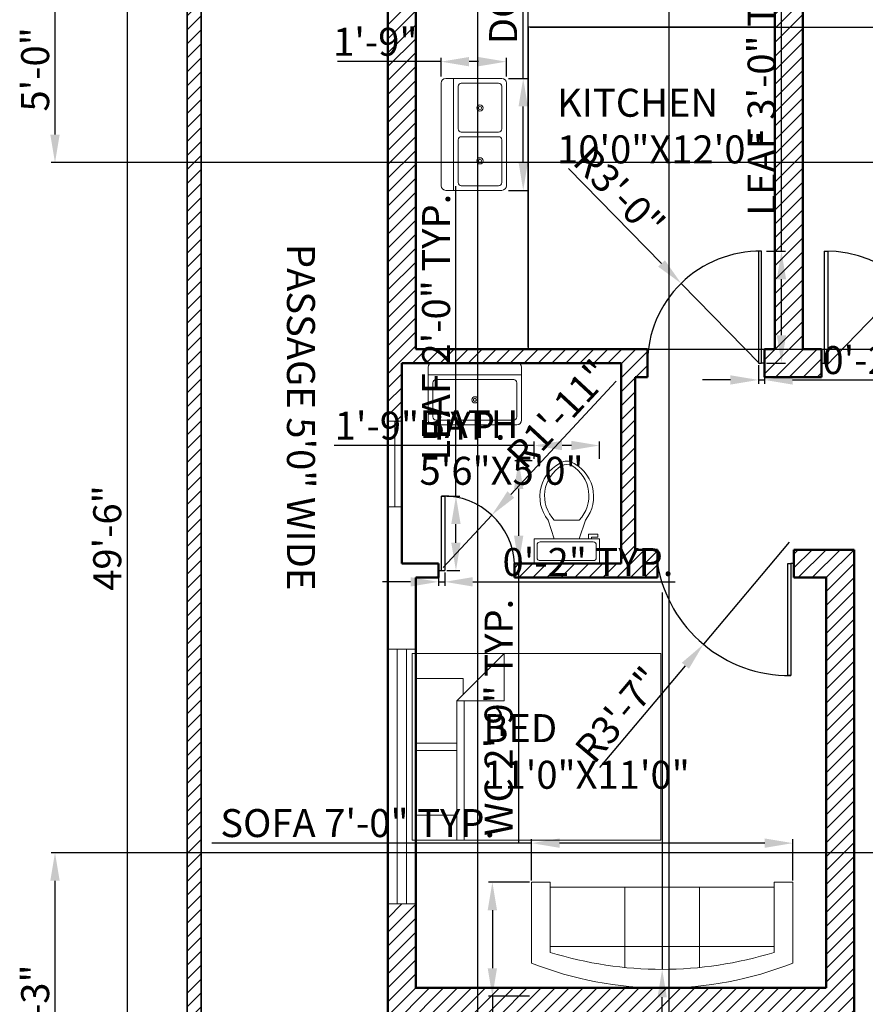
# Model space of a CAD drawing. Units: inches. Extents: x 36184 to 36805, y 18177 to 19069.
# Tile 3 of 5: x 36191 to 36463, y 18560 to 18876. Entities that reach past the tile are written whole.
import ezdxf

# ---------------------------------------------------------------- set-up
doc = ezdxf.new("R2010")
doc.units = ezdxf.units.IN
for name, color, linetype, lineweight in [('A-ANNO-DIMS', 2, 'Continuous', 18), ('A-AREA-IDEN', 7, 'Continuous', 25), ('A-DOOR', 4, 'Continuous', 25), ('A-FLOR-CASE', 9, 'Continuous', 25), ('A-FLOR-FIXT', 9, 'Continuous', 18), ('A-FURN', 8, 'Continuous', 18), ('A-GLAZ', 4, 'Continuous', 18), ('A-WALL', 7, 'Continuous', 50), ('C-PROP', 7, 'Continuous', 35), ('L-SITE-WALL', 7, 'Continuous', 35)]:
    doc.layers.add(name, color=color, linetype=linetype, lineweight=lineweight)
doc.layers.add('A-WALL-PATT', color=244, linetype='Continuous', lineweight=13, true_color=0x991b1e)
doc.styles.get("Standard").update_dxf_attribs({"font": 'arial.ttf'})
doc.dimstyles.new('ISO-25', dxfattribs={"dimtxt": 9, "dimasz": 9, "dimexe": 1.25, "dimexo": 0.625, "dimtad": 1, "dimdec": 1, "dimrnd": 9, "dimlunit": 3, "dimtxsty": 'Standard', "dimcen": 2.5, "dimadec": 0, "dimazin": 0, "dimtfac": 1, "dimtdec": 1, "dimtmove": 0, "dimatfit": 3, "dimfxl": 1, "dimarcsym": 0})

# ---------------------------------------------------------------- blocks, each defined once
blk = doc.blocks.new('Sink-double - 36 in top')
for p, q in [((-18, -4), (18, -4)), ((-0.75, -18.5), (-0.75, -6.5)), ((0.75, -6.5), (0.75, -18.5))]:
    blk.add_line(p, q)
for points in [[(-16.5, 0), (16.5, 0)], [(-18, -19.5), (-18, -1.5)], [(18, -1.5), (18, -19.5)], [(-15.5, -5.5), (-1.75, -5.5)], [(1.75, -5.5), (15.5, -5.5)], [(-16.5, -18.5), (-16.5, -6.5)], [(16.5, -6.5), (16.5, -18.5)], [(16.5, -21), (-16.5, -21)], [(-1.75, -19.5), (-15.5, -19.5)], [(15.5, -19.5), (1.75, -19.5)]]:
    blk.add_lwpolyline(points)
for centre, radius in [((-8.5, -12.5), 1), ((-8.5, -12.5), 0.5), ((8.5, -12.5), 1), ((8.5, -12.5), 0.5)]:
    blk.add_circle(centre, radius)
for centre, radius, start, end in [((-16.5, -1.5), 1.5, 90, 180), ((16.5, -1.5), 1.5, 0, 90), ((-15.5, -6.5), 1, 90, 180), ((-1.75, -6.5), 1, 0, 90), ((1.75, -6.5), 1, 90, 180), ((15.5, -6.5), 1, 0, 90), ((-15.5, -18.5), 1, 180, 270), ((-1.75, -18.5), 1, 270, 0), ((1.75, -18.5), 1, 180, 270), ((15.5, -18.5), 1, 270, 0), ((-16.5, -19.5), 1.5, 180, 270), ((16.5, -19.5), 1.5, 270, 0)]:
    blk.add_arc(centre, radius, start, end)
blk = doc.blocks.new('Sofa - Roundback 7 ft.')
for p, q in [((-12.00002, -32.4421), (-12.00003, -6.5971)), ((11.99997, -32.4421), (11.99998, -6.5971)), ((-36.000027, -34), (-36.000027, -11.4696)), ((35.99998, -34), (35.99998, -11.4696)), ((-35.999844, -13.3819), (35.9998, -13.3819)), ((-36.000027, -32.4421), (35.99998, -32.4421))]:
    blk.add_line(p, q)
for points in [[(-36.000027, -34), (-42.000027, -34), (-42.000027, -8)], [(41.99998, -8), (41.99998, -34), (35.99998, -34)]]:
    blk.add_lwpolyline(points)
for centre, radius, start, end in [((0, -114.25), 114.25, 68.43141, 111.5686), ((-0.00001, -127.1968), 121.1968, 72.72033, 107.2797)]:
    blk.add_arc(centre, radius, start, end)
blk = doc.blocks.new('Bed - Queen')
for p, q in [((0, -80.00003), (0, 0)), ((0, 0), (59.99999, 0)), ((59.99999, 0), (59.99999, -80.00003)), ((7.99999, -1.2), (28.79998, -1.2)), ((7.99999, -14.4), (7.99999, -1.2)), ((28.79998, -1.2), (28.79998, -14.4)), ((31.19999, -1.2), (51.99999, -1.2)), ((31.19999, -14.4), (31.19999, -1.2)), ((51.99999, -1.2), (51.99999, -16.4)), ((0, -14.4), (44.8, -14.4)), ((59.99999, -29.6), (44.8, -14.4)), ((44.8, -14.4), (44.8, -29.6)), ((44.8, -16.8), (0, -16.8)), ((51.99999, -16.4), (46.79936, -16.4)), ((44.8, -29.6), (59.99999, -29.6)), ((59.99999, -80.00003), (0, -80.00003))]:
    blk.add_line(p, q)
blk = doc.blocks.new('Toilet - top')
for p, q in [((9.5, -6), (9.5, -2)), ((-10, -8.5), (-8, -8.5)), ((-10, -9.5), (-10, -8.5)), ((-7, -9.5), (-10, -9.5)), ((-8, -8.5), (-8, -8)), ((-7, -8), (-7, -9.5)), ((-4, -8), (-6, -14)), ((4, -8), (6, -14)), ((4, -14), (-4, -14))]:
    blk.add_line(p, q)
blk.add_lwpolyline([(10.5, -8), (10.5, 0), (-10.5, 0), (-10.5, -8)], close=True)
for points in [[(-9.5, -2), (-9.5, -6)], [(8.5, -1), (-8.5, -1)], [(-8.5, -7), (8.5, -7)]]:
    blk.add_lwpolyline(points)
for centre, radius, start, end in [((-8.62, -1.88), 0.884, 81.8699, 188.1301), ((8.62, -1.88), 0.884, 351.8699, 98.1301), ((-8.62, -6.12), 0.884, 171.8699, 278.1301), ((8.62, -6.12), 0.884, 261.8699, 8.1301), ((3.52, -21.58), 12.17, 141.4691, 247.9714), ((4.2, -21.82), 11.33, 136.3677, 238.9468), ((-3.52, -21.58), 12.17, 292.0284, 38.5307), ((-4.2, -21.82), 11.33, 301.053, 43.6321), ((0, -27.88), 4, 245.7318, 294.2682), ((0, -29), 4, 254.8605, 285.1395)]:
    blk.add_arc(centre, radius, start, end)
blk = doc.blocks.new('Sink-single - 30 in top')
blk.add_line((-15, -3.999996), (15, -3.999996))
for points in [[(-13.5, 0), (13.5, 0)], [(-15, -18.499996), (-15, -1.5)], [(15, -1.5), (15, -18.499996)], [(-12.5, -5.499996), (12.5, -5.499996)], [(-13.5, -17.499996), (-13.5, -6.499996)], [(13.5, -6.499996), (13.5, -17.499996)], [(12.5, -18.499996), (-12.5, -18.499996)], [(13.5, -19.999996), (-13.5, -19.999996)]]:
    blk.add_lwpolyline(points)
for radius in [1, 0.5]:
    blk.add_circle((0, -11.999996), radius)
for centre, radius, start, end in [((-13.5, -1.5), 1.5, 90, 180), ((13.5, -1.5), 1.5, 0, 90), ((-12.5, -6.499996), 1, 90, 180), ((12.5, -6.499996), 1, 0, 90), ((-13.5, -18.499996), 1.5, 180, 270), ((-12.5, -17.499996), 1, 180, 270), ((12.5, -17.499996), 1, 270, 0), ((13.5, -18.499996), 1.5, 270, 0)]:
    blk.add_arc(centre, radius, start, end)
blk = doc.blocks.new('*D14')
at = {"layer": 'A-ANNO-DIMS', "color": 0, "lineweight": -2, "transparency": 16777216}
for p, q in [((36244.69, 19007.3), (36224.73, 19007.3)), ((36225.98, 18998.3), (36225.98, 18420.79)), ((36244.69, 18411.79), (36224.73, 18411.79))]:
    blk.add_line(p, q, dxfattribs=at)
at = {"layer": 'A-ANNO-DIMS', "color": 0, "transparency": 16777216}
for points in [[(36224.48, 18998.3), (36227.48, 18998.3), (36225.98, 19007.3)], [(36224.48, 18420.79), (36227.48, 18420.79), (36225.98, 18411.79)]]:
    blk.add_solid(points, dxfattribs=at)
at = {"layer": 'Defpoints', "color": 0, "transparency": 16777216}
for p in [(36245.31, 19007.3), (36225.98, 18411.79), (36245.31, 18411.79)]:
    blk.add_point(p, dxfattribs=at)
at = {"layer": 'A-ANNO-DIMS', "color": 0, "transparency": 16777216, "insert": (36220.76, 18709.54), "char_height": 9, "attachment_point": 5, "rotation": 90}
blk.add_mtext('49\'-6"', dxfattribs=at)
blk = doc.blocks.new('DOOR-LEAF-24IN')
for p, q in [((1, 0), (1, 24)), ((1, 24), (2, 24)), ((2, 24), (2, 0)), ((0, 0), (1, 0)), ((1, 0), (2, 0))]:
    blk.add_line(p, q)
blk = doc.blocks.new('DOOR-LEAF-36IN')
for p, q in [((1, 36), (0, 36)), ((0, 36), (0, 0)), ((1, 0), (1, 36)), ((0, 0), (1, 0)), ((2, 0), (1, 0))]:
    blk.add_line(p, q)
blk = doc.blocks.new('*D22')
at = {"layer": 'A-ANNO-DIMS', "color": 0, "lineweight": -2, "transparency": 16777216}
for p, q in [((36356.04, 18611.4), (36253.25, 18611.4)), ((36356.04, 18599.43), (36356.04, 18612.65)), ((36431.04, 18611.4), (36365.04, 18611.4)), ((36440.04, 18599.43), (36440.04, 18612.65))]:
    blk.add_line(p, q, dxfattribs=at)
at = {"layer": 'A-ANNO-DIMS', "color": 0, "transparency": 16777216}
for points in [[(36365.04, 18612.9), (36365.04, 18609.9), (36356.04, 18611.4)], [(36431.04, 18612.9), (36431.04, 18609.9), (36440.04, 18611.4)]]:
    blk.add_solid(points, dxfattribs=at)
at = {"layer": 'Defpoints', "color": 0, "transparency": 16777216}
for p in [(36356.04, 18611.4), (36356.04, 18598.8), (36440.04, 18598.8)]:
    blk.add_point(p, dxfattribs=at)
at = {"layer": 'A-ANNO-DIMS', "color": 0, "transparency": 16777216, "insert": (36300.14, 18616.68), "char_height": 9, "attachment_point": 5}
blk.add_mtext('SOFA 7\'-0" TYP.', dxfattribs=at)
blk = doc.blocks.new('*D23')
at = {"layer": 'A-ANNO-DIMS', "color": 0, "lineweight": -2, "transparency": 16777216}
for p, q in [((36355.41, 18598.8), (36342.19, 18598.8)), ((36343.44, 18589.8), (36343.44, 18571.14)), ((36355.41, 18562.14), (36342.19, 18562.14)), ((36343.44, 18562.14), (36343.44, 18476.06))]:
    blk.add_line(p, q, dxfattribs=at)
at = {"layer": 'A-ANNO-DIMS', "color": 0, "transparency": 16777216}
for points in [[(36341.94, 18589.8), (36344.94, 18589.8), (36343.44, 18598.8)], [(36341.94, 18571.14), (36344.94, 18571.14), (36343.44, 18562.14)]]:
    blk.add_solid(points, dxfattribs=at)
at = {"layer": 'Defpoints', "color": 0, "transparency": 16777216}
for p in [(36356.04, 18598.8), (36343.44, 18562.14), (36356.04, 18562.14)]:
    blk.add_point(p, dxfattribs=at)
at = {"layer": 'A-ANNO-DIMS', "color": 0, "transparency": 16777216, "insert": (36338.16, 18514.6), "char_height": 9, "attachment_point": 5, "rotation": 90}
blk.add_mtext('3\'-0 1/2" TYP.', dxfattribs=at)
blk = doc.blocks.new('*D26')
at = {"layer": 'A-ANNO-DIMS', "color": 0, "lineweight": -2, "transparency": 16777216}
for p, q in [((36331.73, 18723.05), (36331.73, 18822.7)), ((36328.75, 18723.05), (36332.98, 18723.05)), ((36331.73, 18708.05), (36331.73, 18714.05)), ((36328.75, 18699.05), (36332.98, 18699.05))]:
    blk.add_line(p, q, dxfattribs=at)
at = {"layer": 'A-ANNO-DIMS', "color": 0, "transparency": 16777216}
for points in [[(36330.23, 18714.05), (36333.23, 18714.05), (36331.73, 18723.05)], [(36330.23, 18708.05), (36333.23, 18708.05), (36331.73, 18699.05)]]:
    blk.add_solid(points, dxfattribs=at)
at = {"layer": 'Defpoints', "color": 0, "transparency": 16777216}
for p in [(36328.13, 18723.05), (36331.73, 18723.05), (36328.13, 18699.05)]:
    blk.add_point(p, dxfattribs=at)
at = {"layer": 'A-ANNO-DIMS', "color": 0, "transparency": 16777216, "insert": (36326.51, 18777.38), "char_height": 9, "attachment_point": 5, "rotation": 90}
blk.add_mtext('LEAF 2\'-0" TYP.', dxfattribs=at)
blk = doc.blocks.new('*D27')
at = {"layer": 'A-ANNO-DIMS', "color": 0, "lineweight": -2, "transparency": 16777216}
for p, q in [((36326.13, 18698.43), (36326.13, 18694.2)), ((36328.13, 18698.43), (36328.13, 18694.2)), ((36317.13, 18695.45), (36308.13, 18695.45)), ((36326.13, 18695.45), (36328.13, 18695.45)), ((36337.13, 18695.45), (36402.24, 18695.45))]:
    blk.add_line(p, q, dxfattribs=at)
at = {"layer": 'A-ANNO-DIMS', "color": 0, "transparency": 16777216}
for points in [[(36317.13, 18696.95), (36317.13, 18693.95), (36326.13, 18695.45)], [(36337.13, 18696.95), (36337.13, 18693.95), (36328.13, 18695.45)]]:
    blk.add_solid(points, dxfattribs=at)
at = {"layer": 'Defpoints', "color": 0, "transparency": 16777216}
for p in [(36326.13, 18699.05), (36328.13, 18699.05), (36328.13, 18695.45)]:
    blk.add_point(p, dxfattribs=at)
at = {"layer": 'A-ANNO-DIMS', "color": 0, "transparency": 16777216, "insert": (36374.18, 18700.67), "char_height": 9, "attachment_point": 5}
blk.add_mtext('0\'-2" TYP.', dxfattribs=at)
blk = doc.blocks.new('*D28')
at = {"layer": 'A-ANNO-DIMS', "color": 0, "lineweight": -2, "transparency": 16777216}
for p, q in [((36436.4, 18801.8), (36436.4, 18901.45)), ((36431.63, 18801.8), (36437.65, 18801.8)), ((36436.4, 18774.8), (36436.4, 18792.8)), ((36431.63, 18765.8), (36437.65, 18765.8))]:
    blk.add_line(p, q, dxfattribs=at)
at = {"layer": 'A-ANNO-DIMS', "color": 0, "transparency": 16777216}
for points in [[(36434.9, 18792.8), (36437.9, 18792.8), (36436.4, 18801.8)], [(36434.9, 18774.8), (36437.9, 18774.8), (36436.4, 18765.8)]]:
    blk.add_solid(points, dxfattribs=at)
at = {"layer": 'Defpoints', "color": 0, "transparency": 16777216}
for p in [(36431, 18801.8), (36436.4, 18801.8), (36431, 18765.8)]:
    blk.add_point(p, dxfattribs=at)
at = {"layer": 'A-ANNO-DIMS', "color": 0, "transparency": 16777216, "insert": (36431.18, 18856.13), "char_height": 9, "attachment_point": 5, "rotation": 90}
blk.add_mtext('LEAF 3\'-0" TYP.', dxfattribs=at)
blk = doc.blocks.new('*D29')
at = {"layer": 'A-ANNO-DIMS', "color": 0, "lineweight": -2, "transparency": 16777216}
for p, q in [((36429, 18765.18), (36429, 18759.15)), ((36431, 18765.18), (36431, 18759.15)), ((36420, 18760.4), (36411, 18760.4)), ((36429, 18760.4), (36431, 18760.4)), ((36440, 18760.4), (36505.11, 18760.4))]:
    blk.add_line(p, q, dxfattribs=at)
at = {"layer": 'A-ANNO-DIMS', "color": 0, "transparency": 16777216}
for points in [[(36420, 18761.9), (36420, 18758.9), (36429, 18760.4)], [(36440, 18761.9), (36440, 18758.9), (36431, 18760.4)]]:
    blk.add_solid(points, dxfattribs=at)
at = {"layer": 'Defpoints', "color": 0, "transparency": 16777216}
for p in [(36429, 18765.8), (36431, 18765.8), (36431, 18760.4)]:
    blk.add_point(p, dxfattribs=at)
at = {"layer": 'A-ANNO-DIMS', "color": 0, "transparency": 16777216, "insert": (36477.06, 18765.62), "char_height": 9, "attachment_point": 5}
blk.add_mtext('0\'-2" TYP.', dxfattribs=at)
blk = doc.blocks.new('*D32')
at = {"layer": 'A-ANNO-DIMS', "color": 0, "lineweight": -2, "transparency": 16777216}
for p, q in [((36356.23, 18734.35), (36350.65, 18734.35)), ((36351.9, 18725.35), (36351.9, 18710.3)), ((36356.23, 18701.3), (36350.65, 18701.3)), ((36351.9, 18701.3), (36351.9, 18611.38))]:
    blk.add_line(p, q, dxfattribs=at)
at = {"layer": 'A-ANNO-DIMS', "color": 0, "transparency": 16777216}
for points in [[(36350.4, 18725.35), (36353.4, 18725.35), (36351.9, 18734.35)], [(36350.4, 18710.3), (36353.4, 18710.3), (36351.9, 18701.3)]]:
    blk.add_solid(points, dxfattribs=at)
at = {"layer": 'Defpoints', "color": 0, "transparency": 16777216}
for p in [(36356.86, 18734.35), (36351.9, 18701.3), (36356.86, 18701.3)]:
    blk.add_point(p, dxfattribs=at)
at = {"layer": 'A-ANNO-DIMS', "color": 0, "transparency": 16777216, "insert": (36346.62, 18651.84), "char_height": 9, "attachment_point": 5, "rotation": 90}
blk.add_mtext('WC 2\'-9" TYP.', dxfattribs=at)
blk = doc.blocks.new('*D33')
at = {"layer": 'A-ANNO-DIMS', "color": 0, "lineweight": -2, "transparency": 16777216}
for p, q in [((36356.86, 18739.31), (36292.59, 18739.31)), ((36356.86, 18734.97), (36356.86, 18740.56)), ((36368.86, 18739.31), (36365.86, 18739.31)), ((36377.86, 18734.97), (36377.86, 18740.56))]:
    blk.add_line(p, q, dxfattribs=at)
at = {"layer": 'A-ANNO-DIMS', "color": 0, "transparency": 16777216}
for points in [[(36365.86, 18740.81), (36365.86, 18737.81), (36356.86, 18739.31)], [(36368.86, 18740.81), (36368.86, 18737.81), (36377.86, 18739.31)]]:
    blk.add_solid(points, dxfattribs=at)
at = {"layer": 'Defpoints', "color": 0, "transparency": 16777216}
for p in [(36356.86, 18739.31), (36356.86, 18734.35), (36377.86, 18734.35)]:
    blk.add_point(p, dxfattribs=at)
at = {"layer": 'A-ANNO-DIMS', "color": 0, "transparency": 16777216, "insert": (36320.22, 18744.53), "char_height": 9, "attachment_point": 5}
blk.add_mtext('1\'-9" TYP.', dxfattribs=at)
blk = doc.blocks.new('*D42')
at = {"layer": 'A-ANNO-DIMS', "color": 0, "lineweight": -2, "transparency": 16777216}
for p, q in [((36353.36, 18857.38), (36353.36, 18979.14)), ((36348.59, 18857.38), (36354.61, 18857.38)), ((36353.36, 18830.38), (36353.36, 18848.38)), ((36348.59, 18821.38), (36354.61, 18821.38))]:
    blk.add_line(p, q, dxfattribs=at)
at = {"layer": 'A-ANNO-DIMS', "color": 0, "transparency": 16777216}
for points in [[(36351.86, 18848.38), (36354.86, 18848.38), (36353.36, 18857.38)], [(36351.86, 18830.38), (36354.86, 18830.38), (36353.36, 18821.38)]]:
    blk.add_solid(points, dxfattribs=at)
at = {"layer": 'Defpoints', "color": 0, "transparency": 16777216}
for p in [(36347.96, 18857.38), (36353.36, 18857.38), (36347.96, 18821.38)]:
    blk.add_point(p, dxfattribs=at)
at = {"layer": 'A-ANNO-DIMS', "color": 0, "transparency": 16777216, "insert": (36348.08, 18922.76), "char_height": 9, "attachment_point": 5, "rotation": 90}
blk.add_mtext('DOUBLE SINK 3\'-0"', dxfattribs=at)
blk = doc.blocks.new('*D43')
at = {"layer": 'A-ANNO-DIMS', "color": 0, "lineweight": -2, "transparency": 16777216}
for p, q in [((36326.96, 18862.78), (36293.64, 18862.78)), ((36326.96, 18858.01), (36326.96, 18864.03)), ((36338.96, 18862.78), (36335.96, 18862.78)), ((36347.96, 18858.01), (36347.96, 18864.03))]:
    blk.add_line(p, q, dxfattribs=at)
at = {"layer": 'A-ANNO-DIMS', "color": 0, "transparency": 16777216}
for points in [[(36335.96, 18864.28), (36335.96, 18861.28), (36326.96, 18862.78)], [(36338.96, 18864.28), (36338.96, 18861.28), (36347.96, 18862.78)]]:
    blk.add_solid(points, dxfattribs=at)
at = {"layer": 'Defpoints', "color": 0, "transparency": 16777216}
for p in [(36326.96, 18862.78), (36326.96, 18857.38), (36347.96, 18857.38)]:
    blk.add_point(p, dxfattribs=at)
at = {"layer": 'A-ANNO-DIMS', "color": 0, "transparency": 16777216, "insert": (36305.8, 18868), "char_height": 9, "attachment_point": 5}
blk.add_mtext('1\'-9"', dxfattribs=at)
blk = doc.blocks.new('*D47')
at = {"layer": 'A-ANNO-DIMS', "color": 0, "lineweight": -2, "transparency": 16777216}
for p, q in [((36519.19, 18608.3), (36201.56, 18608.3)), ((36202.81, 18518.3), (36202.81, 18599.3)), ((36519.19, 18509.3), (36201.56, 18509.3))]:
    blk.add_line(p, q, dxfattribs=at)
at = {"layer": 'A-ANNO-DIMS', "color": 0, "transparency": 16777216}
for points in [[(36201.31, 18599.3), (36204.31, 18599.3), (36202.81, 18608.3)], [(36201.31, 18518.3), (36204.31, 18518.3), (36202.81, 18509.3)]]:
    blk.add_solid(points, dxfattribs=at)
at = {"layer": 'Defpoints', "color": 0, "transparency": 16777216}
for p in [(36202.81, 18608.3), (36519.81, 18608.3), (36519.81, 18509.3)]:
    blk.add_point(p, dxfattribs=at)
at = {"layer": 'A-ANNO-DIMS', "color": 0, "transparency": 16777216, "insert": (36197.59, 18558.8), "char_height": 9, "attachment_point": 5, "rotation": 90}
blk.add_mtext('8\'-3"', dxfattribs=at)
blk = doc.blocks.new('*D49')
at = {"layer": 'A-ANNO-DIMS', "color": 0, "lineweight": -2, "transparency": 16777216}
for p, q in [((36600.19, 18890.3), (36201.56, 18890.3)), ((36202.81, 18839.3), (36202.81, 18881.3)), ((36600.19, 18830.3), (36201.56, 18830.3))]:
    blk.add_line(p, q, dxfattribs=at)
at = {"layer": 'A-ANNO-DIMS', "color": 0, "transparency": 16777216}
for points in [[(36201.31, 18881.3), (36204.31, 18881.3), (36202.81, 18890.3)], [(36201.31, 18839.3), (36204.31, 18839.3), (36202.81, 18830.3)]]:
    blk.add_solid(points, dxfattribs=at)
at = {"layer": 'Defpoints', "color": 0, "transparency": 16777216}
for p in [(36202.81, 18890.3), (36600.81, 18890.3), (36600.81, 18830.3)]:
    blk.add_point(p, dxfattribs=at)
at = {"layer": 'A-ANNO-DIMS', "color": 0, "transparency": 16777216, "insert": (36197.59, 18860.3), "char_height": 9, "attachment_point": 5, "rotation": 90}
blk.add_mtext('5\'-0"', dxfattribs=at)
blk = doc.blocks.new('*D55')
at = {"layer": 'A-ANNO-DIMS', "color": 0, "lineweight": -2, "transparency": 16777216}
for p, q in [((36318.81, 18770.93), (36318.81, 19051.05)), ((36327.81, 19049.8), (36345.96, 19049.8)), ((36354.96, 18770.93), (36354.96, 19051.05))]:
    blk.add_line(p, q, dxfattribs=at)
at = {"layer": 'A-ANNO-DIMS', "color": 0, "transparency": 16777216}
for points in [[(36327.81, 19051.3), (36327.81, 19048.3), (36318.81, 19049.8)], [(36345.96, 19051.3), (36345.96, 19048.3), (36354.96, 19049.8)]]:
    blk.add_solid(points, dxfattribs=at)
at = {"layer": 'Defpoints', "color": 0, "transparency": 16777216}
for p in [(36354.96, 19049.8), (36318.81, 18770.3), (36354.96, 18770.3)]:
    blk.add_point(p, dxfattribs=at)
at = {"layer": 'A-ANNO-DIMS', "color": 0, "transparency": 16777216, "insert": (36336.89, 19055.03), "char_height": 9, "attachment_point": 5}
blk.add_mtext('3\'-0"', dxfattribs=at)
blk = doc.blocks.new('*D56')
at = {"layer": 'A-ANNO-DIMS', "color": 0, "lineweight": -2, "transparency": 16777216}
for p, q in [((36355.59, 18873.92), (36710.68, 18873.92)), ((36709.43, 18864.92), (36709.43, 18779.3)), ((36355.59, 18770.3), (36710.68, 18770.3))]:
    blk.add_line(p, q, dxfattribs=at)
at = {"layer": 'A-ANNO-DIMS', "color": 0, "transparency": 16777216}
for points in [[(36707.93, 18864.92), (36710.93, 18864.92), (36709.43, 18873.92)], [(36707.93, 18779.3), (36710.93, 18779.3), (36709.43, 18770.3)]]:
    blk.add_solid(points, dxfattribs=at)
at = {"layer": 'Defpoints', "color": 0, "transparency": 16777216}
for p in [(36354.96, 18873.92), (36354.96, 18770.3), (36709.43, 18770.3)]:
    blk.add_point(p, dxfattribs=at)
at = {"layer": 'A-ANNO-DIMS', "color": 0, "transparency": 16777216, "insert": (36704.15, 18822.11), "char_height": 9, "attachment_point": 5, "rotation": 90}
blk.add_mtext('8\'-7 1/2"', dxfattribs=at)
blk = doc.blocks.new('*D60')
at = {"layer": 'A-ANNO-DIMS', "color": 0, "lineweight": -2, "transparency": 16777216}
for p, q in [((36338.76, 18403.43), (36338.76, 19051.05)), ((36347.76, 19049.8), (36391.25, 19049.8)), ((36400.25, 18403.43), (36400.25, 19051.05))]:
    blk.add_line(p, q, dxfattribs=at)
at = {"layer": 'A-ANNO-DIMS', "color": 0, "transparency": 16777216}
for points in [[(36347.76, 19051.3), (36347.76, 19048.3), (36338.76, 19049.8)], [(36391.25, 19051.3), (36391.25, 19048.3), (36400.25, 19049.8)]]:
    blk.add_solid(points, dxfattribs=at)
at = {"layer": 'Defpoints', "color": 0, "transparency": 16777216}
for p in [(36400.25, 19049.8), (36338.76, 18402.8), (36400.25, 18402.8)]:
    blk.add_point(p, dxfattribs=at)
at = {"layer": 'A-ANNO-DIMS', "color": 0, "transparency": 16777216, "insert": (36369.51, 19055.08), "char_height": 9, "attachment_point": 5}
blk.add_mtext('5\'-1 1/2"', dxfattribs=at)
blk = doc.blocks.new('*D62')
at = {"layer": 'A-ANNO-DIMS', "color": 0, "lineweight": -2, "transparency": 16777216}
for p, q in [((36438.91, 18708.25), (36411.3, 18675.35)), ((36378, 18635.69), (36405.51, 18668.46))]:
    blk.add_line(p, q, dxfattribs=at)
at = {"layer": 'A-ANNO-DIMS', "color": 0, "transparency": 16777216}
blk.add_solid([(36404.36, 18669.43), (36406.66, 18667.5), (36411.3, 18675.35)], dxfattribs=at)
at = {"layer": 'Defpoints', "color": 0, "transparency": 16777216}
for p in [(36438.91, 18708.25), (36411.3, 18675.35)]:
    blk.add_point(p, dxfattribs=at)
at = {"layer": 'A-ANNO-DIMS', "color": 0, "transparency": 16777216, "insert": (36384.86, 18651.99), "char_height": 9, "attachment_point": 5, "rotation": 49.9864}
blk.add_mtext('R3\'-7"', dxfattribs=at)
blk = doc.blocks.new('*D64')
at = {"layer": 'A-ANNO-DIMS', "color": 0, "lineweight": -2, "transparency": 16777216}
for p, q in [((36512.31, 18828.76), (36482.61, 18797.96)), ((36450.79, 18764.96), (36476.36, 18791.48))]:
    blk.add_line(p, q, dxfattribs=at)
at = {"layer": 'A-ANNO-DIMS', "color": 0, "transparency": 16777216}
blk.add_solid([(36481.53, 18799), (36483.69, 18796.92), (36476.36, 18791.48)], dxfattribs=at)
at = {"layer": 'Defpoints', "color": 0, "transparency": 16777216}
for p in [(36476.36, 18791.48), (36450.79, 18764.96)]:
    blk.add_point(p, dxfattribs=at)
at = {"layer": 'A-ANNO-DIMS', "color": 0, "transparency": 16777216, "insert": (36496.82, 18820.23), "char_height": 9, "attachment_point": 5, "rotation": 46.0444}
blk.add_mtext('R3\'-1"', dxfattribs=at)
blk = doc.blocks.new('*D68')
at = {"layer": 'A-ANNO-DIMS', "color": 0, "lineweight": -2, "transparency": 16777216}
for p, q in [((36383.23, 18760.02), (36349.38, 18723.52)), ((36327.63, 18700.08), (36343.26, 18716.92))]:
    blk.add_line(p, q, dxfattribs=at)
at = {"layer": 'A-ANNO-DIMS', "color": 0, "transparency": 16777216}
blk.add_solid([(36348.28, 18724.54), (36350.48, 18722.5), (36343.26, 18716.92)], dxfattribs=at)
at = {"layer": 'Defpoints', "color": 0, "transparency": 16777216}
for p in [(36343.26, 18716.92), (36327.63, 18700.08)]:
    blk.add_point(p, dxfattribs=at)
at = {"layer": 'A-ANNO-DIMS', "color": 0, "transparency": 16777216, "insert": (36365.6, 18748.57), "char_height": 9, "attachment_point": 5, "rotation": 47.1463}
blk.add_mtext('R1\'-11"', dxfattribs=at)
blk = doc.blocks.new('*D70')
at = {"layer": 'A-ANNO-DIMS', "color": 0, "lineweight": -2, "transparency": 16777216}
for p, q in [((36398.04, 18692), (36398.04, 18570.8)), ((36398.04, 18468.06), (36398.04, 18561.8))]:
    blk.add_line(p, q, dxfattribs=at)
at = {"layer": 'A-ANNO-DIMS', "color": 0, "transparency": 16777216}
blk.add_solid([(36396.54, 18561.8), (36399.54, 18561.8), (36398.04, 18570.8)], dxfattribs=at)
at = {"layer": 'Defpoints', "color": 0, "transparency": 16777216}
for p in [(36398.04, 18692), (36398.04, 18570.8)]:
    blk.add_point(p, dxfattribs=at)
at = {"layer": 'A-ANNO-DIMS', "color": 0, "transparency": 16777216, "insert": (36392.82, 18498.08), "char_height": 9, "attachment_point": 5, "rotation": 89.9998}
blk.add_mtext('7X R10\'-1"', dxfattribs=at)
blk = doc.blocks.new('*D73')
at = {"layer": 'A-ANNO-DIMS', "color": 0, "lineweight": -2, "transparency": 16777216}
for p, q in [((36367.89, 18828.42), (36397.85, 18797.87)), ((36429.5, 18765.61), (36404.15, 18791.45))]:
    blk.add_line(p, q, dxfattribs=at)
at = {"layer": 'A-ANNO-DIMS', "color": 0, "transparency": 16777216}
blk.add_solid([(36398.92, 18798.92), (36396.78, 18796.82), (36404.15, 18791.45)], dxfattribs=at)
at = {"layer": 'Defpoints', "color": 0, "transparency": 16777216}
for p in [(36404.15, 18791.45), (36429.5, 18765.61)]:
    blk.add_point(p, dxfattribs=at)
at = {"layer": 'A-ANNO-DIMS', "color": 0, "transparency": 16777216, "insert": (36383.45, 18820.01), "char_height": 9, "attachment_point": 5, "rotation": 314.4515}
blk.add_mtext('R3\'-0"', dxfattribs=at)

msp = doc.modelspace()

# ---------------------------------------------------------------- hatches: boundary and pattern name
at = {"layer": 'A-WALL-PATT'}
h = msp.add_hatch(dxfattribs=at)
h.set_pattern_fill('ANSI31', color=256)
h.paths.add_polyline_path([(36318.81, 18555.8), (36459.81, 18555.8), (36459.81, 18705.8), (36440.41, 18705.8), (36440.41, 18696.8), (36450.81, 18696.8), (36450.81, 18564.8), (36318.81, 18564.8), (36318.81, 18591.83), (36309.81, 18591.83), (36309.81, 18525.65), (36318.81, 18525.65)], flags=17)
h.paths.add_polyline_path([(36318.81, 18455.41), (36309.81, 18455.41), (36309.81, 18402.8), (36338.76, 18402.8), (36338.76, 18411.8), (36318.81, 18411.8)], flags=17)
h.paths.add_polyline_path([(36423.09, 18411.8), (36400.25, 18411.8), (36400.25, 18402.8), (36423.09, 18402.8)], flags=17)
h.paths.add_polyline_path([(36492.81, 18478.27), (36496.58, 18481.34), (36494.6, 18487.78), (36492.81, 18486.25), (36483.81, 18479.84), (36483.81, 18411.8), (36473.38, 18411.8), (36473.38, 18402.8), (36483.81, 18402.8), (36483.81, 18356.3), (36483.81, 18347.3), (36519.81, 18347.3), (36524.04, 18347.3), (36524.04, 18356.3), (36492.81, 18356.3)], flags=17)
h.paths.add_polyline_path([(36665.31, 18608.3), (36660.81, 18608.3), (36660.81, 18557.3), (36646.76, 18557.3), (36646.76, 18552.8), (36660.81, 18552.8), (36660.81, 18504.8), (36650.24, 18504.8), (36650.24, 18500.3), (36660.81, 18500.3), (36660.81, 18356.3), (36622.58, 18356.3), (36622.58, 18347.3), (36665.31, 18347.3)])
h.paths.add_polyline_path([(36608.31, 18509.3), (36519.81, 18509.3), (36513.55, 18503.95), (36517.84, 18498.69), (36519.81, 18500.3), (36608.31, 18500.3)])
h.paths.add_polyline_path([(36254.31, 18411.79), (36249.81, 18411.79), (36249.81, 19002.8), (36553.31, 19002.8), (36553.31, 19007.3), (36245.31, 19007.3), (36245.31, 18288.82), (36254.31, 18288.82)])
h.paths.add_polyline_path([(36342.97, 18918.8), (36309.81, 18918.8), (36309.81, 18747.12), (36314.31, 18747.12), (36314.31, 18765.8), (36384.81, 18765.8), (36384.81, 18701.3), (36350.57, 18701.3), (36350.57, 18696.8), (36396.53, 18696.8), (36396.53, 18705.8), (36389.31, 18705.8), (36389.31, 18761.3), (36393.31, 18761.3), (36393.31, 18770.3), (36384.81, 18770.3), (36318.81, 18770.3), (36318.81, 18909.8), (36342.97, 18909.8)], flags=17)
h.paths.add_polyline_path([(36469.15, 18918.8), (36403.35, 18918.8), (36403.35, 18909.8), (36434.31, 18909.8), (36434.31, 18770.3), (36431, 18770.3), (36431, 18761.3), (36449.29, 18761.3), (36449.29, 18770.3), (36443.31, 18770.3), (36443.31, 18909.8), (36469.15, 18909.8)], flags=17)
h.paths.add_polyline_path([(36557.81, 18953.44), (36553.31, 18953.44), (36553.31, 18918.8), (36527.35, 18918.8), (36527.35, 18909.8), (36553.31, 18909.8), (36562.16, 18909.8), (36562.16, 18914.3), (36557.81, 18914.3)])
h.paths.add_polyline_path([(36665.31, 19007.3), (36553.31, 19007.3), (36553.31, 19002.8), (36553.31, 18989.93), (36557.81, 18989.93), (36557.81, 19002.8), (36660.81, 19002.8), (36660.81, 18765.8), (36656.73, 18765.8), (36656.73, 18761.3), (36660.81, 18761.3), (36660.81, 18617.3), (36654.49, 18617.3), (36654.49, 18608.3), (36665.31, 18608.3)])
h.paths.add_polyline_path([(36600.81, 18890.3), (36596.31, 18890.3), (36596.31, 18770.3), (36487.63, 18770.3), (36487.63, 18761.3), (36519.81, 18761.3), (36519.81, 18756.26), (36528.81, 18756.26), (36528.81, 18761.3), (36634.81, 18761.3), (36634.81, 18765.8), (36600.81, 18765.8), (36600.81, 18825.8), (36660.81, 18825.8), (36660.81, 18830.3), (36600.81, 18830.3)])
h.paths.add_polyline_path([(36600.81, 18914.3), (36596.31, 18914.3), (36591.43, 18914.3), (36591.43, 18909.8), (36596.31, 18909.8), (36596.31, 18890.3), (36660.81, 18890.3), (36660.81, 18894.8), (36600.81, 18894.8)], flags=17)
h.paths.add_polyline_path([(36623.57, 18617.3), (36528.81, 18617.3), (36528.81, 18717.38), (36519.81, 18717.38), (36519.81, 18608.3), (36608.31, 18608.3), (36608.31, 18603.13), (36617.31, 18603.13), (36617.31, 18608.3), (36623.57, 18608.3)])
h.paths.add_polyline_path([(36602.02, 18898.95), (36663.11, 18898.95), (36663.11, 18913.37), (36602.02, 18913.37)], flags=25)

# ---------------------------------------------------------------- linework, layer by layer
at = {"layer": 'A-DOOR'}
for centre, radius, start, end in [((36429.5, 18765.61), 36.2, 89.2085, 179.6946), ((36450.79, 18764.96), 36.85, 1.3121, 90.7775), ((36327.63, 18700.08), 22.98, 3.047, 91.2469), ((36438.91, 18708.25), 42.95, 189.3065, 270.667)]:
    msp.add_arc(centre, radius, start, end, dxfattribs=at)
at = {"layer": 'A-FLOR-CASE'}
for p, q in [((36434.31, 18873.92), (36354.96, 18873.92)), ((36354.96, 18873.92), (36354.96, 18770.3))]:
    msp.add_line(p, q, dxfattribs=at)
at = {"layer": 'A-GLAZ'}
for p, q in [((36314.31, 18747.12), (36309.81, 18747.12)), ((36312.06, 18747.12), (36312.06, 18719.58)), ((36314.31, 18719.58), (36309.81, 18719.58)), ((36318.81, 18673.84), (36309.81, 18673.84)), ((36312.81, 18673.84), (36312.81, 18591.83)), ((36315.81, 18673.84), (36315.81, 18591.83)), ((36318.81, 18591.83), (36309.81, 18591.83))]:
    msp.add_line(p, q, dxfattribs=at)
at = {"layer": 'A-WALL'}
for p, q in [((36309.81, 18918.8), (36309.81, 18402.8)), ((36318.81, 18909.8), (36318.81, 18770.3)), ((36434.31, 18770.3), (36434.31, 18909.8)), ((36443.31, 18770.3), (36443.31, 18909.8)), ((36318.81, 18770.3), (36384.81, 18770.3)), ((36393.31, 18770.3), (36384.81, 18770.3)), ((36393.31, 18770.3), (36393.31, 18761.3)), ((36434.31, 18770.3), (36431, 18770.3)), ((36431, 18770.3), (36431, 18761.3)), ((36449.29, 18770.3), (36443.31, 18770.3)), ((36449.29, 18770.3), (36449.29, 18761.3)), ((36314.31, 18765.8), (36384.81, 18765.8)), ((36314.31, 18765.8), (36314.31, 18701.3)), ((36384.81, 18765.8), (36384.81, 18701.3)), ((36389.31, 18761.3), (36389.31, 18705.8)), ((36393.31, 18761.3), (36389.31, 18761.3)), ((36449.29, 18761.3), (36431, 18761.3)), ((36396.53, 18705.8), (36389.31, 18705.8)), ((36396.53, 18705.8), (36396.53, 18696.8)), ((36459.81, 18705.8), (36440.41, 18705.8)), ((36440.41, 18705.8), (36440.41, 18696.8)), ((36459.81, 18705.8), (36459.81, 18555.8)), ((36326.13, 18701.3), (36314.31, 18701.3)), ((36326.13, 18701.3), (36326.13, 18696.8)), ((36384.81, 18701.3), (36350.57, 18701.3)), ((36350.57, 18701.3), (36350.57, 18696.8)), ((36318.81, 18696.8), (36318.81, 18564.8)), ((36326.13, 18696.8), (36318.81, 18696.8)), ((36396.53, 18696.8), (36350.57, 18696.8)), ((36450.81, 18696.8), (36440.41, 18696.8)), ((36450.81, 18696.8), (36450.81, 18564.8)), ((36450.81, 18564.8), (36318.81, 18564.8))]:
    msp.add_line(p, q, dxfattribs=at)
at = {"layer": 'C-PROP'}
msp.add_line((36245.31, 19007.3), (36245.31, 18227.3), dxfattribs=at)
at = {"layer": 'L-SITE-WALL'}
msp.add_line((36249.81, 19002.8), (36249.81, 18411.79), dxfattribs=at)

# ---------------------------------------------------------------- block references
at = {"layer": 'A-DOOR'}
for name, p in [('DOOR-LEAF-36IN', (36429, 18765.8)), ('DOOR-LEAF-24IN', (36326.13, 18699.05))]:
    msp.add_blockref(name, p, dxfattribs=at)
at = {"layer": 'A-DOOR', "extrusion": (0, 0, -1), "zscale": -1}
msp.add_blockref('DOOR-LEAF-36IN', (-36451.29, 18765.8), dxfattribs=at)
at = {"layer": 'A-DOOR', "extrusion": (0, 0, -1), "zscale": -1, "rotation": 180}
msp.add_blockref('DOOR-LEAF-36IN', (-36438.41, 18701.3), dxfattribs=at)
at = {"layer": 'A-FLOR-FIXT'}
for name, p, rotation in [('Sink-double - 36 in top', (36326.96, 18839.38), 90), ('Toilet - top', (36367.36, 18701.3), 180)]:
    msp.add_blockref(name, p, dxfattribs=dict(at, rotation=rotation))
msp.add_blockref('Sink-single - 30 in top', (36337.82, 18765.99), dxfattribs=at)
at = {"layer": 'A-FURN'}
for name, p, rotation in [('Bed - Queen', (36317.61, 18612.4), 89.99999999999999), ('Sofa - Roundback 7 ft.', (36398.04, 18564.8), 180)]:
    msp.add_blockref(name, p, dxfattribs=dict(at, rotation=rotation))

# ---------------------------------------------------------------- texts
at = {"layer": 'A-AREA-IDEN', "char_height": 9, "attachment_point": 1}
for s, width, insert in [('KITCHEN\\P10\'0"X12\'0"', 58.2547, (36364.26, 18854.06)), ('BATH\\P5\'6"X5\'0"', 79.9285, (36320.02, 18750.67)), ('BED \\P11\'0"X11\'0"', 83.9217, (36340.54, 18652.89))]:
    msp.add_mtext_dynamic_manual_height_columns(s, width=width, gutter_width=12.5, heights=[0], dxfattribs=dict(at, insert=insert))
at = {"layer": 'A-AREA-IDEN', "insert": (36286.4, 18804.15), "char_height": 9, "attachment_point": 1, "rotation": 270}
msp.add_mtext_dynamic_manual_height_columns('PASSAGE 5\'0" WIDE', width=233.2566, gutter_width=12.5, heights=[0], dxfattribs=at)

# ---------------------------------------------------------------- dimensions: what is measured, and where the dimension line sits
at = {"layer": 'A-ANNO-DIMS'}
for base, p1, p2, picture, middle in [((36400.25, 19049.8), (36338.76, 18402.8), (36400.25, 18402.8), '*D60', (36369.51, 19055.08)), ((36354.9601, 19049.8021), (36318.8117, 18770.3021), (36354.9601, 18770.3021), '*D55', (36336.8859, 19055.0254))]:
    dim = msp.add_linear_dim(base=base, p1=p1, p2=p2, dimstyle='ISO-25', override={"dimdec": 1, "dimlfac": 1, "dimrnd": 0, "dimzin": 1, "dimdsep": 46, "dimlunit": 4, "dimfrac": 2}, dxfattribs=at)
    dim.commit()
    dim.dimension.update_dxf_attribs({"geometry": picture, "text_midpoint": middle})
for base, p1, p2, angle, override, picture, middle in [((36225.98, 18411.79), (36245.31, 19007.3), (36245.31, 18411.79), 90, {"dimclrd": 0, "dimclre": 0, "dimclrt": 0}, '*D14', (36220.76, 18709.54)), ((36202.81, 18890.3), (36600.81, 18830.3), (36600.81, 18890.3), 90, {"dimdec": 1, "dimlfac": 1, "dimrnd": 0, "dimzin": 1, "dimdsep": 46, "dimlunit": 4, "dimfrac": 2}, '*D49', (36197.59, 18860.3)), ((36326.96, 18862.78), (36347.96, 18857.38), (36326.96, 18857.38), 180, {"dimdec": 1, "dimlfac": 1, "dimrnd": 0, "dimzin": 1, "dimdsep": 46, "dimlunit": 4, "dimfrac": 2}, '*D43', (36305.8, 18868)), ((36709.43, 18770.3), (36354.96, 18873.92), (36354.96, 18770.3), 90, {"dimdec": 1, "dimlfac": 1, "dimrnd": 0, "dimzin": 1, "dimdsep": 46, "dimlunit": 4, "dimfrac": 2}, '*D56', (36704.15, 18822.11)), ((36202.81, 18608.3), (36519.81, 18509.3), (36519.81, 18608.3), 90, {"dimdec": 1, "dimlfac": 1, "dimrnd": 0, "dimzin": 1, "dimdsep": 46, "dimlunit": 4, "dimfrac": 2}, '*D47', (36197.59, 18558.8))]:
    dim = msp.add_linear_dim(base=base, p1=p1, p2=p2, angle=angle, dimstyle='ISO-25', override=override, dxfattribs=at)
    dim.commit()
    dim.dimension.update_dxf_attribs({"geometry": picture, "text_midpoint": middle})
for base, p1, p2, angle, text, picture, middle in [((36353.36, 18857.38), (36347.96, 18821.38), (36347.96, 18857.38), 90, 'DOUBLE SINK <>', '*D42', (36348.08, 18922.76)), ((36436.4, 18801.8), (36431, 18765.8), (36431, 18801.8), 90, 'LEAF <> TYP.', '*D28', (36431.18, 18856.13)), ((36331.73, 18723.05), (36328.13, 18699.05), (36328.13, 18723.05), 90, 'LEAF <> TYP.', '*D26', (36326.51, 18777.38)), ((36356.86, 18739.31), (36377.86, 18734.35), (36356.86, 18734.35), 180, '<> TYP.', '*D33', (36320.22, 18744.53)), ((36351.899, 18701.3021), (36356.856, 18734.3484), (36356.856, 18701.3021), 270, 'WC <> TYP.', '*D32', (36346.6206, 18651.8432)), ((36356.04, 18611.4), (36440.04, 18598.8), (36356.04, 18598.8), 180, 'SOFA <> TYP.', '*D22', (36300.14, 18616.68)), ((36343.44, 18562.14), (36356.04, 18598.8), (36356.04, 18562.14), 270, '<> TYP.', '*D23', (36338.16, 18514.6))]:
    dim = msp.add_linear_dim(base=base, p1=p1, p2=p2, angle=angle, text=text, dimstyle='ISO-25', override={"dimdec": 1, "dimlfac": 1, "dimrnd": 0, "dimzin": 1, "dimdsep": 46, "dimlunit": 4, "dimfrac": 2}, dxfattribs=at)
    dim.commit()
    dim.dimension.update_dxf_attribs({"geometry": picture, "text_midpoint": middle})
for center, mpoint, picture, middle in [((36429.5, 18765.61), (36404.15, 18791.45), '*D73', (36383.45, 18820.01)), ((36450.79, 18764.96), (36476.36, 18791.48), '*D64', (36496.82, 18820.23)), ((36327.63, 18700.08), (36343.26, 18716.92), '*D68', (36365.6, 18748.57)), ((36438.9103, 18708.2475), (36411.2958, 18675.3538), '*D62', (36384.8598, 18651.9873))]:
    dim = msp.add_radius_dim(center=center, mpoint=mpoint, dimstyle='ISO-25', override={"dimdec": 1, "dimlfac": 1, "dimrnd": 0, "dimzin": 1, "dimdsep": 46, "dimlunit": 4, "dimfrac": 2}, dxfattribs=at)
    dim.commit()
    dim.dimension.update_dxf_attribs({"geometry": picture, "text_midpoint": middle})
for base, p1, p2, picture, middle in [((36431, 18760.4), (36429, 18765.8), (36431, 18765.8), '*D29', (36477.06, 18765.62)), ((36328.13, 18695.45), (36326.13, 18699.05), (36328.13, 18699.05), '*D27', (36374.18, 18700.67))]:
    dim = msp.add_linear_dim(base=base, p1=p1, p2=p2, text='<> TYP.', dimstyle='ISO-25', override={"dimdec": 1, "dimlfac": 1, "dimrnd": 0, "dimzin": 1, "dimdsep": 46, "dimlunit": 4, "dimfrac": 2}, dxfattribs=at)
    dim.commit()
    dim.dimension.update_dxf_attribs({"geometry": picture, "text_midpoint": middle})
dim = msp.add_radius_dim(center=(36398.04, 18692), mpoint=(36398.04, 18570.8), text='7X <>', dimstyle='ISO-25', override={"dimdec": 1, "dimlfac": 1, "dimrnd": 0, "dimzin": 1, "dimdsep": 46, "dimlunit": 4, "dimfrac": 2}, dxfattribs=at)
dim.commit()
dim.dimension.update_dxf_attribs({"geometry": '*D70', "text_midpoint": (36398.04, 18498.08), "dimtype": 164})

doc.saveas('drawing.dxf')
